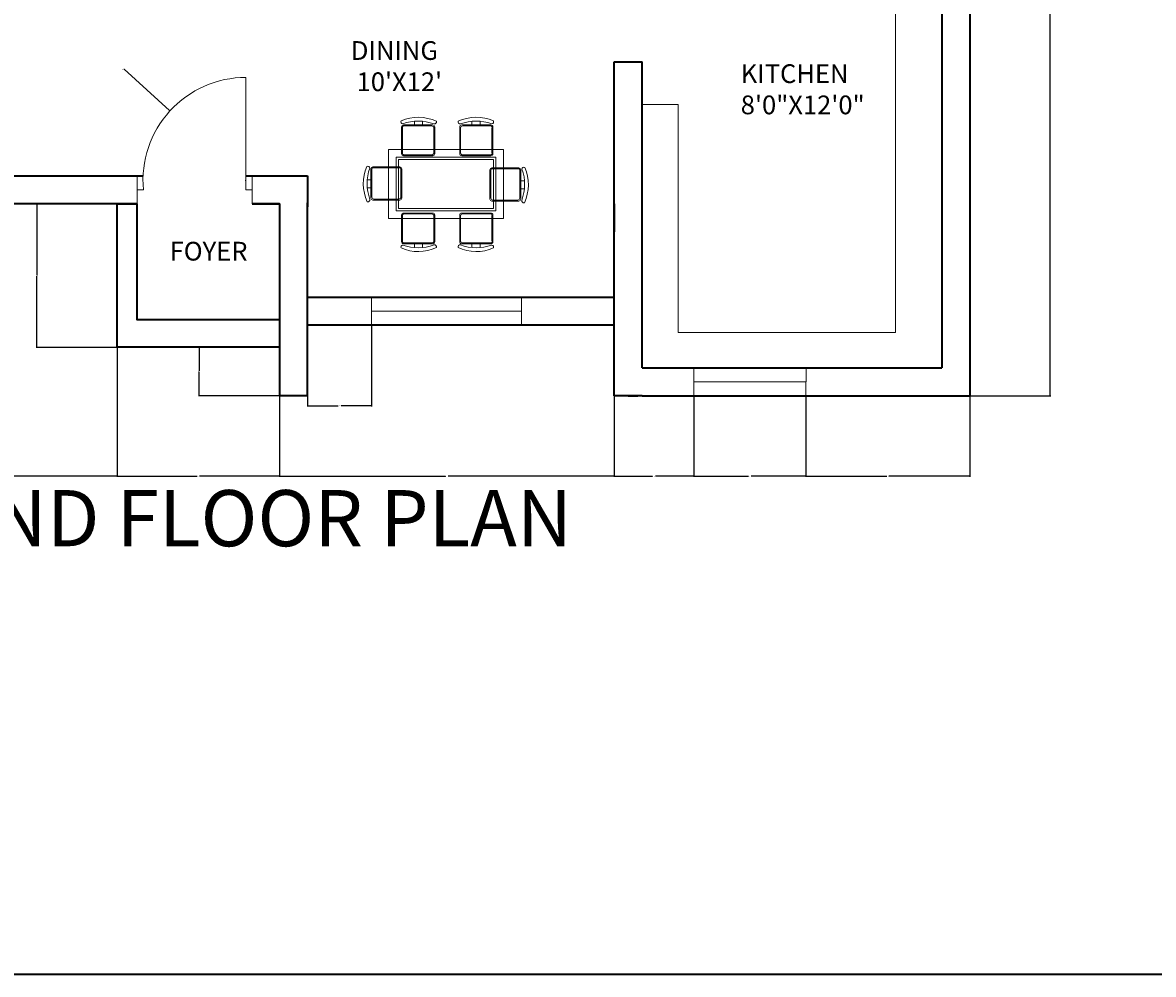
# Model space of a CAD drawing. Units: inches. Extents: x 2067 to 3463, y 1605 to 2723.
# Tile 4 of 10: x 2403 to 2765, y 1605 to 1910. Entities that reach past the tile are written whole.
import ezdxf

# ---------------------------------------------------------------- set-up
doc = ezdxf.new("R2010")
doc.units = ezdxf.units.IN
for name, color, linetype, lineweight in [('A-ANNO-DIMS', 2, 'Continuous', 18), ('A-ANNO-TEXT', 7, 'Continuous', 35), ('A-ANNO-TTLB', 7, 'Continuous', 35), ('A-AREA-IDEN', 7, 'Continuous', 18), ('A-DOOR', 3, 'Continuous', 18), ('A-FLOR-CASE', 8, 'Continuous', 18), ('A-FURN', 8, 'Continuous', 13), ('A-GLAZ', 4, 'Continuous', 18), ('A-WALL', 7, 'Continuous', 35)]:
    doc.layers.add(name, color=color, linetype=linetype, lineweight=lineweight)
doc.styles.get("Standard").update_dxf_attribs({"font": 'arial.ttf'})
doc.dimstyles.get("Standard").update_dxf_attribs({"dimtxt": 0.18, "dimasz": 0.18, "dimexe": 0.18, "dimexo": 0.0625, "dimgap": 0.09, "dimtad": 0, "dimtih": 1, "dimtoh": 1, "dimdec": 4, "dimzin": 0, "dimdsep": 46, "dimtxsty": 'Standard', "dimcen": 0.09, "dimadec": 0, "dimazin": 0, "dimtfac": 1, "dimtdec": 4, "dimtofl": 0, "dimtmove": 0, "dimatfit": 3, "dimfxl": 1, "dimtolj": 1, "dimtzin": 0, "dimarcsym": 0})

# ---------------------------------------------------------------- blocks, each defined once
blk = doc.blocks.new('*D29')
at = {"layer": 'A-ANNO-DIMS', "color": 0, "lineweight": -2, "transparency": 16777216}
for p, q in [((2706.51, 2158.23), (2732.43, 2158.23)), ((2732.25, 2158.05), (2732.25, 1974.66)), ((2732.25, 1790.91), (2732.25, 1974.3)), ((2706.51, 1790.73), (2732.43, 1790.73))]:
    blk.add_line(p, q, dxfattribs=at)
at = {"layer": 'A-ANNO-DIMS', "color": 0, "transparency": 16777216}
for points in [[(2732.22, 2158.05), (2732.28, 2158.05), (2732.25, 2158.23)], [(2732.22, 1790.91), (2732.28, 1790.91), (2732.25, 1790.73)]]:
    blk.add_solid(points, dxfattribs=at)
at = {"layer": 'Defpoints', "color": 0, "transparency": 16777216}
for p in [(2706.45, 2158.23), (2732.25, 2158.23), (2706.45, 1790.73)]:
    blk.add_point(p, dxfattribs=at)
at = {"layer": 'A-ANNO-DIMS', "color": 0, "transparency": 16777216, "insert": (2732.25, 1974.48), "char_height": 0.18, "attachment_point": 5}
blk.add_mtext('\\A1;367.5', dxfattribs=at)
blk = doc.blocks.new('*D34')
at = {"layer": 'A-ANNO-DIMS', "color": 0, "lineweight": -2, "transparency": 16777216}
for p, q in [((2433.19, 1852.22), (2407.27, 1852.22)), ((2407.45, 1852.04), (2407.45, 1829.42)), ((2407.45, 1806.43), (2407.45, 1829.05)), ((2433.19, 1806.25), (2407.27, 1806.25))]:
    blk.add_line(p, q, dxfattribs=at)
at = {"layer": 'A-ANNO-DIMS', "color": 0, "transparency": 16777216}
for points in [[(2407.42, 1852.04), (2407.48, 1852.04), (2407.45, 1852.22)], [(2407.42, 1806.43), (2407.48, 1806.43), (2407.45, 1806.25)]]:
    blk.add_solid(points, dxfattribs=at)
at = {"layer": 'Defpoints', "color": 0, "transparency": 16777216}
for p in [(2407.45, 1852.22), (2433.25, 1852.22), (2433.25, 1806.25)]:
    blk.add_point(p, dxfattribs=at)
at = {"layer": 'A-ANNO-DIMS', "color": 0, "transparency": 16777216, "insert": (2407.45, 1829.23), "char_height": 0.18, "attachment_point": 5}
blk.add_mtext('\\A1;45.96', dxfattribs=at)
blk = doc.blocks.new('*D35')
at = {"layer": 'A-ANNO-DIMS', "color": 0, "lineweight": -2, "transparency": 16777216}
for p, q in [((2485.17, 1806.25), (2459.26, 1806.25)), ((2459.44, 1806.07), (2459.44, 1798.67)), ((2459.44, 1790.91), (2459.44, 1798.31)), ((2485.17, 1790.73), (2459.26, 1790.73))]:
    blk.add_line(p, q, dxfattribs=at)
at = {"layer": 'A-ANNO-DIMS', "color": 0, "transparency": 16777216}
for points in [[(2459.41, 1806.07), (2459.47, 1806.07), (2459.44, 1806.25)], [(2459.41, 1790.91), (2459.47, 1790.91), (2459.44, 1790.73)]]:
    blk.add_solid(points, dxfattribs=at)
at = {"layer": 'Defpoints', "color": 0, "transparency": 16777216}
for p in [(2459.44, 1806.25), (2485.24, 1806.25), (2485.24, 1790.73)]:
    blk.add_point(p, dxfattribs=at)
at = {"layer": 'A-ANNO-DIMS', "color": 0, "transparency": 16777216, "insert": (2459.44, 1798.49), "char_height": 0.18, "attachment_point": 5}
blk.add_mtext('\\A1;15.522', dxfattribs=at)
blk = doc.blocks.new('*D36')
at = {"layer": 'A-ANNO-DIMS', "color": 0, "lineweight": -2, "transparency": 16777216}
for p, q in [((2268.95, 1852.15), (2268.95, 1764.75)), ((2433.25, 1806.19), (2433.25, 1764.75)), ((2269.13, 1764.93), (2350.71, 1764.93)), ((2433.07, 1764.93), (2351.49, 1764.93))]:
    blk.add_line(p, q, dxfattribs=at)
at = {"layer": 'A-ANNO-DIMS', "color": 0, "transparency": 16777216}
for points in [[(2269.13, 1764.96), (2269.13, 1764.9), (2268.95, 1764.93)], [(2433.07, 1764.96), (2433.07, 1764.9), (2433.25, 1764.93)]]:
    blk.add_solid(points, dxfattribs=at)
at = {"layer": 'Defpoints', "color": 0, "transparency": 16777216}
for p in [(2268.95, 1852.22), (2433.25, 1806.25), (2433.25, 1764.93)]:
    blk.add_point(p, dxfattribs=at)
at = {"layer": 'A-ANNO-DIMS', "color": 0, "transparency": 16777216, "insert": (2351.1, 1764.93), "char_height": 0.18, "attachment_point": 5}
blk.add_mtext('\\A1;164.3', dxfattribs=at)
blk = doc.blocks.new('*D37')
at = {"layer": 'A-ANNO-DIMS', "color": 0, "lineweight": -2, "transparency": 16777216}
for p, q in [((2433.25, 1806.19), (2433.25, 1764.75)), ((2485.24, 1790.67), (2485.24, 1764.75)), ((2433.43, 1764.93), (2458.85, 1764.93)), ((2485.06, 1764.93), (2459.64, 1764.93))]:
    blk.add_line(p, q, dxfattribs=at)
at = {"layer": 'A-ANNO-DIMS', "color": 0, "transparency": 16777216}
for points in [[(2433.43, 1764.96), (2433.43, 1764.9), (2433.25, 1764.93)], [(2485.06, 1764.96), (2485.06, 1764.9), (2485.24, 1764.93)]]:
    blk.add_solid(points, dxfattribs=at)
at = {"layer": 'Defpoints', "color": 0, "transparency": 16777216}
for p in [(2433.25, 1806.25), (2485.24, 1790.73), (2485.24, 1764.93)]:
    blk.add_point(p, dxfattribs=at)
at = {"layer": 'A-ANNO-DIMS', "color": 0, "transparency": 16777216, "insert": (2459.24, 1764.93), "char_height": 0.18, "attachment_point": 5}
blk.add_mtext('\\A1;51.98', dxfattribs=at)
blk = doc.blocks.new('*D38')
at = {"layer": 'A-ANNO-DIMS', "color": 0, "lineweight": -2, "transparency": 16777216}
for p, q in [((2485.24, 1790.67), (2485.24, 1764.75)), ((2592.45, 1790.67), (2592.45, 1764.75)), ((2485.42, 1764.93), (2538.4, 1764.93)), ((2592.27, 1764.93), (2539.28, 1764.93))]:
    blk.add_line(p, q, dxfattribs=at)
at = {"layer": 'A-ANNO-DIMS', "color": 0, "transparency": 16777216}
for points in [[(2485.42, 1764.96), (2485.42, 1764.9), (2485.24, 1764.93)], [(2592.27, 1764.96), (2592.27, 1764.9), (2592.45, 1764.93)]]:
    blk.add_solid(points, dxfattribs=at)
at = {"layer": 'Defpoints', "color": 0, "transparency": 16777216}
for p in [(2485.24, 1790.73), (2592.45, 1790.73), (2592.45, 1764.93)]:
    blk.add_point(p, dxfattribs=at)
at = {"layer": 'A-ANNO-DIMS', "color": 0, "transparency": 16777216, "insert": (2538.84, 1764.93), "char_height": 0.18, "attachment_point": 5}
blk.add_mtext('\\A1;107.21', dxfattribs=at)
blk = doc.blocks.new('*D39')
at = {"layer": 'A-ANNO-DIMS', "color": 0, "lineweight": -2, "transparency": 16777216}
for p, q in [((2592.45, 1790.67), (2592.45, 1764.75)), ((2617.98, 1790.67), (2617.98, 1764.75)), ((2592.63, 1764.93), (2604.75, 1764.93)), ((2617.8, 1764.93), (2605.68, 1764.93))]:
    blk.add_line(p, q, dxfattribs=at)
at = {"layer": 'A-ANNO-DIMS', "color": 0, "transparency": 16777216}
for points in [[(2592.63, 1764.96), (2592.63, 1764.9), (2592.45, 1764.93)], [(2617.8, 1764.96), (2617.8, 1764.9), (2617.98, 1764.93)]]:
    blk.add_solid(points, dxfattribs=at)
at = {"layer": 'Defpoints', "color": 0, "transparency": 16777216}
for p in [(2592.45, 1790.73), (2617.98, 1790.73), (2617.98, 1764.93)]:
    blk.add_point(p, dxfattribs=at)
at = {"layer": 'A-ANNO-DIMS', "color": 0, "transparency": 16777216, "insert": (2605.21, 1764.93), "char_height": 0.18, "attachment_point": 5}
blk.add_mtext('\\A1;25.533', dxfattribs=at)
blk = doc.blocks.new('*D40')
at = {"layer": 'A-ANNO-DIMS', "color": 0, "lineweight": -2, "transparency": 16777216}
for p, q in [((2617.98, 1790.67), (2617.98, 1764.75)), ((2653.95, 1790.67), (2653.95, 1764.75)), ((2618.16, 1764.93), (2635.57, 1764.93)), ((2653.77, 1764.93), (2636.36, 1764.93))]:
    blk.add_line(p, q, dxfattribs=at)
at = {"layer": 'A-ANNO-DIMS', "color": 0, "transparency": 16777216}
for points in [[(2618.16, 1764.96), (2618.16, 1764.9), (2617.98, 1764.93)], [(2653.77, 1764.96), (2653.77, 1764.9), (2653.95, 1764.93)]]:
    blk.add_solid(points, dxfattribs=at)
at = {"layer": 'Defpoints', "color": 0, "transparency": 16777216}
for p in [(2617.98, 1790.73), (2653.95, 1790.73), (2653.95, 1764.93)]:
    blk.add_point(p, dxfattribs=at)
at = {"layer": 'A-ANNO-DIMS', "color": 0, "transparency": 16777216, "insert": (2635.96, 1764.93), "char_height": 0.18, "attachment_point": 5}
blk.add_mtext('\\A1;35.97', dxfattribs=at)
blk = doc.blocks.new('*D41')
at = {"layer": 'A-ANNO-DIMS', "color": 0, "lineweight": -2, "transparency": 16777216}
for p, q in [((2653.95, 1790.67), (2653.95, 1764.75)), ((2706.45, 1790.67), (2706.45, 1764.75)), ((2654.13, 1764.93), (2679.87, 1764.93)), ((2706.27, 1764.93), (2680.52, 1764.93))]:
    blk.add_line(p, q, dxfattribs=at)
at = {"layer": 'A-ANNO-DIMS', "color": 0, "transparency": 16777216}
for points in [[(2654.13, 1764.96), (2654.13, 1764.9), (2653.95, 1764.93)], [(2706.27, 1764.96), (2706.27, 1764.9), (2706.45, 1764.93)]]:
    blk.add_solid(points, dxfattribs=at)
at = {"layer": 'Defpoints', "color": 0, "transparency": 16777216}
for p in [(2653.95, 1790.73), (2706.45, 1790.73), (2706.45, 1764.93)]:
    blk.add_point(p, dxfattribs=at)
at = {"layer": 'A-ANNO-DIMS', "color": 0, "transparency": 16777216, "insert": (2680.2, 1764.93), "char_height": 0.18, "attachment_point": 5}
blk.add_mtext('\\A1;52.5', dxfattribs=at)
blk = doc.blocks.new('*D43')
at = {"layer": 'A-ANNO-DIMS', "color": 0, "lineweight": -2, "transparency": 16777216}
for p, q in [((2494.24, 1813.26), (2494.24, 1787.34)), ((2514.75, 1813.26), (2514.75, 1787.34)), ((2494.42, 1787.52), (2504.03, 1787.52)), ((2514.57, 1787.52), (2504.96, 1787.52))]:
    blk.add_line(p, q, dxfattribs=at)
at = {"layer": 'A-ANNO-DIMS', "color": 0, "transparency": 16777216}
for points in [[(2494.42, 1787.55), (2494.42, 1787.49), (2494.24, 1787.52)], [(2514.57, 1787.55), (2514.57, 1787.49), (2514.75, 1787.52)]]:
    blk.add_solid(points, dxfattribs=at)
at = {"layer": 'Defpoints', "color": 0, "transparency": 16777216}
for p in [(2494.24, 1813.32), (2514.75, 1813.32), (2494.24, 1787.52)]:
    blk.add_point(p, dxfattribs=at)
at = {"layer": 'A-ANNO-DIMS', "color": 0, "transparency": 16777216, "insert": (2504.49, 1787.52), "char_height": 0.18, "attachment_point": 5}
blk.add_mtext('\\A1;20.515', dxfattribs=at)
blk = doc.blocks.new('*D102')
at = {"layer": 'A-ANNO-DIMS', "color": 0, "lineweight": -2, "transparency": 16777216}
for p, q in [((2435.31, 1895.31), (2435.49, 1895.31)), ((2435.49, 1895.31), (2449.98, 1882.09)), ((2474.39, 1859.72), (2474.57, 1859.72)), ((2474.48, 1859.63), (2474.48, 1859.81))]:
    blk.add_line(p, q, dxfattribs=at)
at = {"layer": 'A-ANNO-DIMS', "color": 0, "transparency": 16777216}
blk.add_solid([(2450, 1882.11), (2449.96, 1882.06), (2450.11, 1881.97)], dxfattribs=at)
at = {"layer": 'Defpoints', "color": 0, "transparency": 16777216}
for p in [(2450.11, 1881.97), (2474.48, 1859.72)]:
    blk.add_point(p, dxfattribs=at)
at = {"layer": 'A-ANNO-DIMS', "color": 0, "transparency": 16777216, "insert": (2435, 1895.31), "char_height": 0.18, "attachment_point": 5}
blk.add_mtext('\\A1;R33', dxfattribs=at)

msp = doc.modelspace()

# ---------------------------------------------------------------- linework, layer by layer
at = {"layer": 'A-ANNO-TTLB'}
msp.add_lwpolyline([(2067.2624, 2722.6321), (3463.3053, 2722.6321), (3463.3053, 1605.3918), (2067.2624, 1605.3918)], close=True, dxfattribs=at)
at = {"layer": 'A-DOOR'}
for p, q in [((2474.4815, 1856.7171), (2474.4815, 1892.7171)), ((2439.6214, 1861.2171), (2439.6214, 1852.2171)), ((2476.4815, 1852.2171), (2476.4815, 1861.2171)), ((2476.4815, 1861.2171), (2476.4815, 1856.7171)), ((2439.6214, 1852.2171), (2439.6214, 1856.7171)), ((2439.6214, 1856.7171), (2441.6214, 1856.7171)), ((2476.4815, 1856.7171), (2474.4815, 1856.7171))]:
    msp.add_line(p, q, dxfattribs=at)
msp.add_arc((2474.4815, 1859.7201), 32.997, 90, 185.221564, dxfattribs=at)
at = {"layer": 'A-FLOR-CASE'}
for p, q in [((2682.5961, 1811.0125), (2682.5961, 1943.7309)), ((2601.4477, 1884.0112), (2612.9658, 1884.0112)), ((2612.9658, 1884.0112), (2612.9658, 1811.0125)), ((2612.9658, 1811.0125), (2682.5961, 1811.0125))]:
    msp.add_line(p, q, dxfattribs=at)
at = {"layer": 'A-FURN'}
for points in [[(2524.7218, 1877.8935, -0.17580919), (2534.7621, 1877.8175, 0.57839206), (2535.5227, 1878.6538, 0.21452438), (2524.1894, 1878.8059, 0.55201397), (2524.7218, 1877.8935, -0.06507904)], [(2534.3361, 1877.4905), (2525.0151, 1877.4905, 0.41421356), (2524.363, 1876.8384), (2524.363, 1868.2679, 0.41421356), (2525.0151, 1867.6158), (2534.3361, 1867.6158, 0.41421356), (2534.9882, 1868.2679), (2534.9882, 1876.8384, 0.41421356), (2534.3361, 1877.4905)], [(2531.0621, 1877.4905), (2531.0621, 1878.6693, -0.06475861)], [(2543.2147, 1877.8175, -0.57839206), (2542.4541, 1878.6538, -0.21452438), (2553.7874, 1878.8059, -0.55201397), (2553.2549, 1877.8935, 0.1758092), (2543.2147, 1877.8175)], [(2552.9617, 1877.4905, -0.41421356), (2553.6138, 1876.8384), (2553.6138, 1868.2679, -0.41421356), (2552.9617, 1867.6158), (2543.6407, 1867.6158, -0.41421356), (2542.9885, 1868.2679), (2542.9885, 1876.8384, -0.41421356), (2543.6407, 1877.4905), (2552.9617, 1877.4905)], [(2546.9147, 1877.4905), (2546.9147, 1878.6693, 0.06475861)], [(2514.2178, 1853.6478, -0.57839206), (2513.3814, 1852.8872, -0.21452438), (2513.2294, 1864.2205, -0.55201397), (2514.1418, 1863.6881, 0.17580937), (2514.2178, 1853.6478)], [(2514.5447, 1863.3948, -0.41421356), (2515.1968, 1864.0469), (2523.7674, 1864.0469, -0.41421356), (2524.4195, 1863.3948), (2524.4195, 1854.0738, -0.41421356), (2523.7674, 1853.4217), (2515.1968, 1853.4217, -0.41421356), (2514.5447, 1854.0738), (2514.5447, 1863.3948)], [(2562.5437, 1863.0756, 0.41421356), (2561.8916, 1863.7277), (2553.3211, 1863.7277, 0.41421356), (2552.669, 1863.0756), (2552.669, 1853.7545, 0.41421356), (2553.3211, 1853.1024), (2561.8916, 1853.1024, 0.41421356), (2562.5437, 1853.7545), (2562.5437, 1863.0756)], [(2562.9467, 1863.3688, -0.17580919), (2562.8706, 1853.3286, 0.57839206), (2563.707, 1852.5679, 0.21452438), (2563.8591, 1863.9013, 0.55201397), (2562.9467, 1863.3688, -0.06507904)], [(2514.5447, 1857.3478), (2513.3659, 1857.3478, 0.06475861)], [(2562.5437, 1857.0286), (2563.7225, 1857.0286, -0.06475861)], [(2534.3361, 1839.3925), (2525.0151, 1839.3925, -0.41421356), (2524.363, 1840.0446), (2524.363, 1848.6151, -0.41421356), (2525.0151, 1849.2672), (2534.3361, 1849.2672, -0.41421356), (2534.9882, 1848.6151), (2534.9882, 1840.0446, -0.41421356), (2534.3361, 1839.3925)], [(2552.9617, 1839.3925, 0.41421356), (2553.6138, 1840.0446), (2553.6138, 1848.6151, 0.41421356), (2552.9617, 1849.2672), (2543.6407, 1849.2672, 0.41421356), (2542.9885, 1848.6151), (2542.9885, 1840.0446, 0.41421356), (2543.6407, 1839.3925), (2552.9617, 1839.3925)], [(2534.7621, 1839.0656, -0.57839206), (2535.5227, 1838.2292, -0.21452438), (2524.1894, 1838.0771, -0.55201397), (2524.7218, 1838.9895, 0.17580929), (2534.7621, 1839.0656)], [(2531.0621, 1839.3925), (2531.0621, 1838.2137, 0.06475861)], [(2553.2549, 1838.9895, -0.17580928), (2543.2147, 1839.0656, 0.57839206), (2542.4541, 1838.2292, 0.21452438), (2553.7874, 1838.0771, 0.55201397), (2553.2549, 1838.9895, -0.06507904)], [(2546.9147, 1839.3925), (2546.9147, 1838.2137, -0.06475861)]]:
    msp.add_lwpolyline(points, format="xyb", dxfattribs=at)
for points in [[(2525.019, 1877.1967), (2534.0423, 1877.1967, -0.41421356), (2534.6945, 1876.5446), (2534.6945, 1868.5617, -0.41421356), (2534.0423, 1867.9096), (2525.019, 1867.9096, -0.51206948), (2524.6568, 1868.5617), (2524.6568, 1876.5446, -0.51206948)], [(2552.9577, 1877.1967), (2543.9344, 1877.1967, 0.41421356), (2543.2823, 1876.5446), (2543.2823, 1868.5617, 0.41421356), (2543.9344, 1867.9096), (2552.9577, 1867.9096, 0.51206948), (2553.32, 1868.5617), (2553.32, 1876.5446, 0.51206948)], [(2514.8385, 1863.3908), (2514.8385, 1854.3675, 0.41421356), (2515.4906, 1853.7154), (2523.4736, 1853.7154, 0.41421356), (2524.1257, 1854.3675), (2524.1257, 1863.3908, 0.51206948), (2523.4736, 1863.7531), (2515.4906, 1863.7531, 0.51206948)], [(2562.2499, 1863.0716), (2562.2499, 1854.0483, -0.41421356), (2561.5978, 1853.3962), (2553.6148, 1853.3962, -0.41421356), (2552.9627, 1854.0483), (2552.9627, 1863.0716, -0.51206948), (2553.6148, 1863.4339), (2561.5978, 1863.4339, -0.51206948)], [(2525.019, 1839.6863), (2534.0423, 1839.6863, 0.41421356), (2534.6945, 1840.3384), (2534.6945, 1848.3213, 0.41421356), (2534.0423, 1848.9735), (2525.019, 1848.9735, 0.51206948), (2524.6568, 1848.3213), (2524.6568, 1840.3384, 0.51206948)], [(2552.9577, 1839.6863), (2543.9344, 1839.6863, -0.41421356), (2543.2823, 1840.3384), (2543.2823, 1848.3213, -0.41421356), (2543.9344, 1848.9735), (2552.9577, 1848.9735, -0.51206948), (2553.32, 1848.3213), (2553.32, 1840.3384, -0.51206948)]]:
    msp.add_lwpolyline(points, format="xyb", close=True, dxfattribs=at)
for points in [[(2528.453, 1878.6908), (2528.453, 1877.4905)], [(2549.5238, 1878.6908), (2549.5238, 1877.4905)], [(2513.3445, 1859.9569), (2514.5447, 1859.9569)], [(2563.7439, 1859.6376), (2562.5437, 1859.6376)], [(2528.453, 1838.1923), (2528.453, 1839.3925)], [(2549.5238, 1838.1923), (2549.5238, 1839.3925)]]:
    msp.add_lwpolyline(points, dxfattribs=at)
for points in [[(2520.1623, 1869.6187), (2557.0247, 1869.6187), (2557.0247, 1847.5013), (2520.1623, 1847.5013)], [(2522.6198, 1867.1612), (2554.5672, 1867.1612), (2554.5672, 1849.9588), (2522.6198, 1849.9588)], [(2523.3571, 1866.4239), (2553.8299, 1866.4239), (2553.8299, 1850.696), (2523.3571, 1850.696)]]:
    msp.add_lwpolyline(points, close=True, dxfattribs=at)
at = {"layer": 'A-GLAZ'}
for p, q in [((2514.7509, 1822.3185), (2514.7509, 1813.3185)), ((2562.7509, 1817.8185), (2562.7509, 1822.3185)), ((2562.7509, 1822.3185), (2562.7509, 1813.3185)), ((2514.7509, 1813.3185), (2514.7509, 1817.8185)), ((2514.7509, 1817.8185), (2550.7509, 1817.8185)), ((2550.7509, 1817.8185), (2562.7509, 1817.8185)), ((2617.981, 1799.7309), (2617.981, 1790.7309)), ((2653.981, 1799.7309), (2653.9477, 1790.7309)), ((2653.981, 1795.2309), (2653.981, 1799.7309)), ((2617.981, 1790.7309), (2617.981, 1795.2309)), ((2617.981, 1795.2309), (2653.981, 1795.2309))]:
    msp.add_line(p, q, dxfattribs=at)
at = {"layer": 'A-WALL'}
for p, q in [((2706.4477, 2158.2309), (2706.4477, 1790.7309)), ((2697.4477, 1943.7309), (2697.4477, 1799.7309)), ((2592.4477, 1790.7309), (2592.4477, 1897.7296)), ((2592.4477, 1897.7296), (2601.4477, 1897.7296)), ((2601.4477, 1799.7309), (2601.4477, 1897.7296)), ((2277.9477, 1861.2171), (2441.5184, 1861.2171)), ((2474.4815, 1861.2171), (2485.2361, 1861.2171)), ((2485.2361, 1861.2171), (2494.2361, 1861.2171)), ((2494.2361, 1861.2171), (2494.2361, 1851.2359)), ((2439.6214, 1852.2171), (2277.9477, 1852.2171)), ((2485.2361, 1852.2171), (2476.4815, 1852.2171)), ((2485.2361, 1852.2171), (2485.2361, 1790.7309)), ((2494.2361, 1790.7309), (2494.2361, 1852.528)), ((2592.4477, 1852.2309), (2592.4477, 1843.2309)), ((2494.2361, 1813.3185), (2494.2361, 1822.3185)), ((2494.2361, 1822.3185), (2592.4477, 1822.3185)), ((2592.4477, 1813.3185), (2494.2361, 1813.3185)), ((2601.4477, 1799.7309), (2697.4477, 1799.7309)), ((2494.2361, 1790.7309), (2485.2361, 1790.7309)), ((2601.4477, 1790.7309), (2592.4477, 1790.7309)), ((2596.9477, 1790.7309), (2600.0965, 1790.7309)), ((2601.4477, 1790.7309), (2706.4477, 1790.7309))]:
    msp.add_line(p, q, dxfattribs=at)
for points in [[(2476.4815, 1852.2171), (2485.2361, 1852.2171), (2485.2361, 1806.2527), (2433.2522, 1806.2527), (2433.2522, 1852.2171), (2439.6214, 1852.2171)], [(2476.4815, 1852.2171), (2485.2361, 1852.2171), (2485.2361, 1815.0381), (2439.6214, 1815.0381), (2439.6214, 1852.2171)]]:
    msp.add_lwpolyline(points, dxfattribs=at)

# ---------------------------------------------------------------- texts
at = {"layer": 'A-ANNO-TEXT', "insert": (2324.4644, 1760.5241), "char_height": 18, "attachment_point": 1}
msp.add_mtext_dynamic_manual_height_columns('GROUND FLOOR PLAN', width=395.878396, gutter_width=12.5, heights=[0], dxfattribs=at)
at = {"layer": 'A-AREA-IDEN', "char_height": 6, "attachment_point": 1}
for s, width, insert in [("DINING\\P 10'X12'", 112.029053, (2508.1142, 1904.3265)), ('KITCHEN\\P8\'0"X12\'0"', 113.326628, (2633.0424, 1896.9125)), ('FOYER', 40.254073, (2450.0171, 1840.0478))]:
    msp.add_mtext_dynamic_manual_height_columns(s, width=width, gutter_width=12.5, heights=[0], dxfattribs=dict(at, insert=insert))

# ---------------------------------------------------------------- dimensions: what is measured, and where the dimension line sits
at = {"layer": 'A-ANNO-DIMS'}
for base, p1, p2, angle, override, picture, middle in [((2732.2477, 2158.2309), (2706.4477, 1790.7309), (2706.4477, 2158.2309), 90, {"dimdec": 1, "dimlfac": 1, "dimrnd": 0, "dimzin": 0, "dimdsep": 46, "dimlunit": 2}, '*D29', (2732.2477, 1974.4809)), ((2407.4522, 1852.2171), (2433.2522, 1806.2527), (2433.2522, 1852.2171), 90, {"dimdec": 2, "dimlfac": 1, "dimrnd": 0, "dimzin": 0, "dimdsep": 46, "dimlunit": 2}, '*D34', (2407.4522, 1829.2349)), ((2494.2361, 1787.5185), (2514.7509, 1813.3185), (2494.2361, 1813.3185), 180, {"dimdec": 3, "dimlfac": 1, "dimrnd": 0, "dimzin": 0, "dimdsep": 46, "dimlunit": 2}, '*D43', (2504.4935, 1787.5185)), ((2459.4361, 1806.2527), (2485.2361, 1790.7309), (2485.2361, 1806.2527), 90, {"dimdec": 3, "dimlfac": 1, "dimrnd": 0, "dimzin": 0, "dimdsep": 46, "dimlunit": 2}, '*D35', (2459.4361, 1798.4918))]:
    dim = msp.add_linear_dim(base=base, p1=p1, p2=p2, angle=angle, dimstyle='Standard', override=override, dxfattribs=at)
    dim.commit()
    dim.dimension.update_dxf_attribs({"geometry": picture, "text_midpoint": middle})
dim = msp.add_radius_dim(center=(2474.4815, 1859.7201), mpoint=(2450.1105, 1881.9656), dimstyle='Standard', override={"dimdec": 0, "dimlfac": 1, "dimrnd": 0, "dimzin": 0, "dimdsep": 46, "dimlunit": 2}, dxfattribs=at)
dim.commit()
dim.dimension.update_dxf_attribs({"geometry": '*D102', "text_midpoint": (2435.0029, 1895.3128), "dimtype": 164})
for base, p1, p2, override, picture, middle in [((2433.2522, 1764.9309), (2268.9477, 1852.2171), (2433.2522, 1806.2527), {"dimdec": 1, "dimlfac": 1, "dimrnd": 0, "dimzin": 0, "dimdsep": 46, "dimlunit": 2}, '*D36', (2351.0999, 1764.9309)), ((2485.2361, 1764.9309), (2433.2522, 1806.2527), (2485.2361, 1790.7309), {"dimdec": 2, "dimlfac": 1, "dimrnd": 0, "dimzin": 0, "dimdsep": 46, "dimlunit": 2}, '*D37', (2459.2441, 1764.9309)), ((2592.4477, 1764.9309), (2485.2361, 1790.7309), (2592.4477, 1790.7309), {"dimdec": 2, "dimlfac": 1, "dimrnd": 0, "dimzin": 0, "dimdsep": 46, "dimlunit": 2}, '*D38', (2538.8419, 1764.9309)), ((2617.981, 1764.9309), (2592.4477, 1790.7309), (2617.981, 1790.7309), {"dimdec": 3, "dimlfac": 1, "dimrnd": 0, "dimzin": 0, "dimdsep": 46, "dimlunit": 2}, '*D39', (2605.2143, 1764.9309)), ((2653.9477, 1764.9309), (2617.981, 1790.7309), (2653.9477, 1790.7309), {"dimdec": 2, "dimlfac": 1, "dimrnd": 0, "dimzin": 0, "dimdsep": 46, "dimlunit": 2}, '*D40', (2635.9643, 1764.9309)), ((2706.4477, 1764.9309), (2653.9477, 1790.7309), (2706.4477, 1790.7309), {"dimdec": 1, "dimlfac": 1, "dimrnd": 0, "dimzin": 0, "dimdsep": 46, "dimlunit": 2}, '*D41', (2680.1977, 1764.9309))]:
    dim = msp.add_linear_dim(base=base, p1=p1, p2=p2, dimstyle='Standard', override=override, dxfattribs=at)
    dim.commit()
    dim.dimension.update_dxf_attribs({"geometry": picture, "text_midpoint": middle})

doc.saveas('drawing.dxf')
